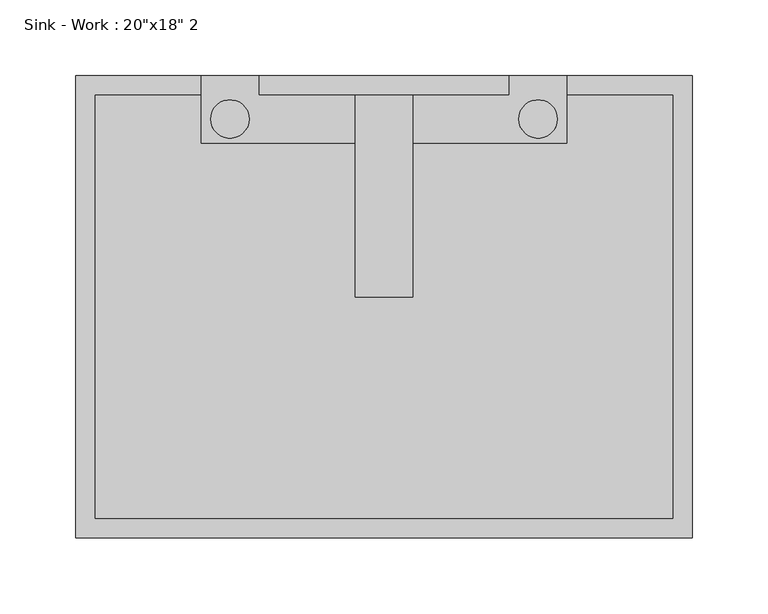
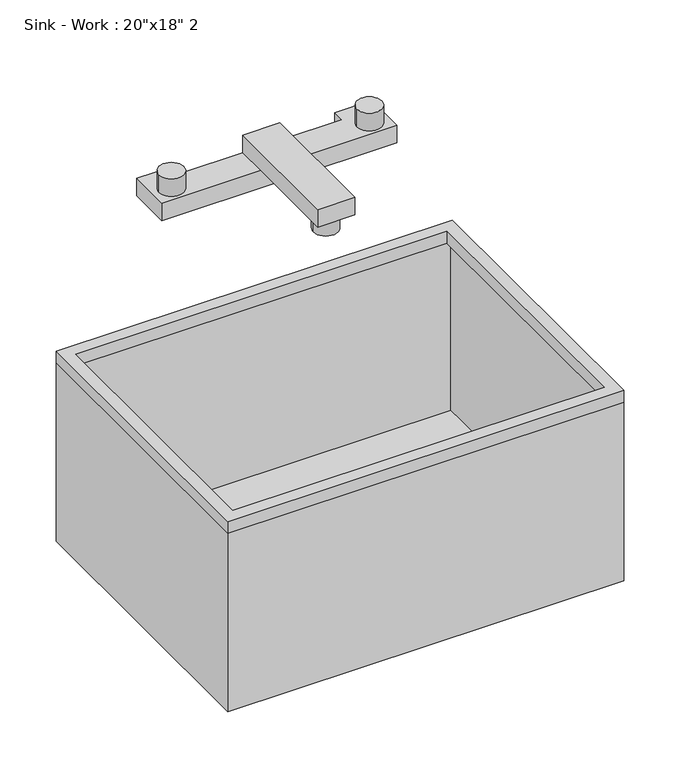
"""IFC4 building model written with IfcOpenShell, lengths in millimetres: flow terminal geometry."""

from ifc_helpers import new_model, si_unit, point, frame, frame_2d, origin, origin_with_axes, place, context, project, spatial, polyline, circle_curve, trimmed, segment, composite_curve, outline, extrude, faceted_brep, source, transform, mapped, element, save
from ifc_brep_helpers import plane_surface, cylinder_surface, advanced_brep


def flow_terminal_7145266d(model_context):
    return source(origin(), model_context, "Body", "SolidModel", [
        extrude(outline(polyline([(203.2, 0.0), (203.2, -304.8), (-203.2, -304.8), (-203.2, 0.0), (203.2, 0.0)]), holes=[polyline([(190.5, -12.7), (-190.5, -12.7), (-190.5, -292.1), (190.5, -292.1), (190.5, -12.7)])]), frame((0.0, 0.0, 193.675), z_axis=(0.0, 0.0, 1.0), x_axis=(1.0, 0.0, 0.0)), (0.0, 0.0, 1.0), 12.7),
        faceted_brep([(203.2, 0.0, 193.675), (-203.2, 0.0, 193.675), (-203.2, -304.8, 193.675), (203.2, -304.8, 193.675), (200.025, -3.175, 193.675), (200.025, -301.625, 193.675), (-200.025, -301.625, 193.675), (-200.025, -3.175, 193.675), (203.2, 0.0, 0.0), (203.2, -304.8, 0.0), (-203.2, -304.8, 0.0), (-203.2, 0.0, 0.0), (200.025, -3.175, 3.175), (200.025, -301.625, 3.175), (-200.025, -301.625, 3.175), (-200.025, -3.175, 3.175)], [[[0, 1, 2, 3], [4, 5, 6, 7]], [[8, 9, 10, 11]], [[1, 0, 8, 11]], [[2, 1, 11, 10]], [[3, 2, 10, 9]], [[0, 3, 9, 8]], [[5, 4, 12, 13]], [[6, 5, 13, 14]], [[7, 6, 14, 15]], [[4, 7, 15, 12]], [[13, 12, 15, 14]]]),
        extrude(outline(composite_curve([segment(trimmed(circle_curve(frame_2d((0.0, -127.0)), 25.4), [point((-25.4, -127.0))], [point((25.4, -127.0))], False, "CARTESIAN"), True, "CONTINUOUS"), segment(trimmed(circle_curve(frame_2d((0.0, -127.0)), 25.4), [point((25.4, -127.0))], [point((-25.4, -127.0))], False, "CARTESIAN"), True, "CONTINUOUS")], self_intersect=False)), origin_with_axes(), (0.0, 0.0, 1.0), 3.175),
        advanced_brep(
        [(19.05, -12.7, 384.175), (-19.05, -12.7, 384.175), (-19.05, -146.05, 384.175), (19.05, -146.05, 384.175), (19.05, -146.05, 365.125), (-19.05, -146.05, 365.125), (-19.05, -44.45, 365.125), (19.05, -44.45, 365.125), (-12.7, -127.0, 365.125), (12.7, -127.0, 365.125), (19.05, -12.7, 365.125), (82.55, -12.7, 365.125), (82.55, -12.7, 346.075), (-82.55, -12.7, 346.075), (-82.55, -12.7, 365.125), (-19.05, -12.7, 365.125), (-12.7, -127.0, 346.075), (12.7, -127.0, 346.075), (-82.55, 0.0, 365.125), (-120.65, 0.0, 365.125), (-120.65, -44.45, 365.125), (-88.9, -28.575, 365.125), (-114.3, -28.575, 365.125), (120.65, -44.45, 365.125), (120.65, 0.0, 365.125), (82.55, 0.0, 365.125), (114.3, -28.575, 365.125), (88.9, -28.575, 365.125), (-82.55, 0.0, 346.075), (82.55, 0.0, 346.075), (120.65, 0.0, 346.075), (120.65, -44.45, 346.075), (-120.65, -44.45, 346.075), (-120.65, 0.0, 346.075), (-114.3, -28.575, 384.175), (-88.9, -28.575, 384.175), (88.9, -28.575, 384.175), (114.3, -28.575, 384.175)],
        [
            (0, 1),
            (1, 2),
            (2, 3),
            (3, 0),
            (4, 5),
            (5, 6),
            (6, 7),
            (7, 4),
            (8, 9, circle_curve(frame((0.0, -127.0, 365.125), z_axis=(0.0, 0.0, 1.0), x_axis=(1.0, 0.0, 0.0)), 12.7)),
            (9, 8, circle_curve(frame((0.0, -127.0, 365.125), z_axis=(0.0, 0.0, 1.0), x_axis=(1.0, 0.0, 0.0)), 12.7)),
            (0, 10),
            (10, 11),
            (11, 12),
            (12, 13),
            (13, 14),
            (14, 15),
            (15, 1),
            (15, 6),
            (5, 2),
            (4, 3),
            (7, 10),
            (16, 17, circle_curve(frame((0.0, -127.0, 346.075), z_axis=(0.0, 0.0, -1.0), x_axis=(1.0, 0.0, 0.0)), 12.7)),
            (17, 16, circle_curve(frame((0.0, -127.0, 346.075), z_axis=(0.0, 0.0, -1.0), x_axis=(1.0, 0.0, 0.0)), 12.7)),
            (17, 9),
            (8, 16),
            (18, 19),
            (19, 20),
            (20, 6),
            (14, 18),
            (21, 22, circle_curve(frame((-101.6, -28.575, 365.125), z_axis=(0.0, 0.0, -1.0), x_axis=(1.0, 0.0, 0.0)), 12.7)),
            (22, 21, circle_curve(frame((-101.6, -28.575, 365.125), z_axis=(0.0, 0.0, -1.0), x_axis=(1.0, 0.0, 0.0)), 12.7)),
            (23, 24),
            (24, 25),
            (25, 11),
            (7, 23),
            (26, 27, circle_curve(frame((101.6, -28.575, 365.125), z_axis=(0.0, 0.0, -1.0), x_axis=(1.0, 0.0, 0.0)), 12.7)),
            (27, 26, circle_curve(frame((101.6, -28.575, 365.125), z_axis=(0.0, 0.0, -1.0), x_axis=(1.0, 0.0, 0.0)), 12.7)),
            (28, 13),
            (12, 29),
            (29, 30),
            (30, 31),
            (31, 32),
            (32, 33),
            (33, 28),
            (18, 28),
            (33, 19),
            (32, 20),
            (31, 23),
            (30, 24),
            (29, 25),
            (34, 35, circle_curve(frame((-101.6, -28.575, 384.175), z_axis=(0.0, 0.0, 1.0), x_axis=(1.0, 0.0, 0.0)), 12.7)),
            (35, 34, circle_curve(frame((-101.6, -28.575, 384.175), z_axis=(0.0, 0.0, 1.0), x_axis=(1.0, 0.0, 0.0)), 12.7)),
            (36, 37, circle_curve(frame((101.6, -28.575, 384.175), z_axis=(0.0, 0.0, 1.0), x_axis=(1.0, 0.0, 0.0)), 12.7)),
            (37, 36, circle_curve(frame((101.6, -28.575, 384.175), z_axis=(0.0, 0.0, 1.0), x_axis=(1.0, 0.0, 0.0)), 12.7)),
            (34, 22),
            (21, 35),
            (36, 27),
            (26, 37),
        ],
        [
            plane_surface(frame((-19.05, -12.7, 384.175), z_axis=(0.0, 0.0, 1.0), x_axis=(-1.0, 0.0, 0.0))),
            plane_surface(frame((-19.05, -12.7, 365.125), z_axis=(0.0, 0.0, -1.0), x_axis=(1.0, 0.0, 0.0))),
            plane_surface(frame((19.05, -12.7, 384.175), z_axis=(0.0, 1.0, 0.0), x_axis=(0.0, 0.0, -1.0))),
            plane_surface(frame((-19.05, -12.7, 384.175), z_axis=(-1.0, 0.0, 0.0), x_axis=(0.0, 0.0, -1.0))),
            plane_surface(frame((-19.05, -146.05, 384.175), z_axis=(0.0, -1.0, 0.0), x_axis=(0.0, 0.0, -1.0))),
            plane_surface(frame((19.05, -146.05, 384.175), z_axis=(1.0, 0.0, 0.0), x_axis=(0.0, 0.0, -1.0))),
            plane_surface(frame((12.7, -127.0, 346.075), z_axis=(0.0, 0.0, -1.0), x_axis=(0.0, -1.0, 0.0))),
            cylinder_surface(frame((0.0, -127.0, 346.075), z_axis=(0.0, 0.0, 1.0), x_axis=(1.0, 0.0, 0.0)), 12.7),
            plane_surface(frame((-120.65, 0.0, 365.125), z_axis=(0.0, 0.0, 1.0), x_axis=(-1.0, 0.0, 0.0))),
            plane_surface(frame((-120.65, 0.0, 346.075), z_axis=(0.0, 0.0, -1.0), x_axis=(1.0, 0.0, 0.0))),
            plane_surface(frame((-82.55, 0.0, 365.125), z_axis=(0.0, 1.0, 0.0), x_axis=(0.0, 0.0, -1.0))),
            plane_surface(frame((-120.65, 0.0, 365.125), z_axis=(-1.0, 0.0, 0.0), x_axis=(0.0, 0.0, -1.0))),
            plane_surface(frame((-120.65, -44.45, 365.125), z_axis=(0.0, -1.0, 0.0), x_axis=(0.0, 0.0, -1.0))),
            plane_surface(frame((120.65, -44.45, 365.125), z_axis=(1.0, 0.0, 0.0), x_axis=(0.0, 0.0, -1.0))),
            plane_surface(frame((120.65, 0.0, 365.125), z_axis=(0.0, 1.0, 0.0), x_axis=(0.0, 0.0, -1.0))),
            plane_surface(frame((82.55, 0.0, 365.125), z_axis=(-1.0, 0.0, 0.0), x_axis=(0.0, 0.0, -1.0))),
            plane_surface(frame((-82.55, -12.7, 365.125), z_axis=(1.0, 0.0, 0.0), x_axis=(0.0, 0.0, -1.0))),
            plane_surface(frame((-88.9, -28.575, 384.175), z_axis=(0.0, 0.0, 1.0), x_axis=(0.0, 1.0, 0.0))),
            cylinder_surface(frame((-101.6, -28.575, 365.125), z_axis=(0.0, 0.0, 1.0), x_axis=(1.0, 0.0, 0.0)), 12.7),
            cylinder_surface(frame((101.6, -28.575, 0.0), z_axis=(0.0, 0.0, 1.0), x_axis=(1.0, 0.0, 0.0)), 12.7),
        ],
        [
            (0, [[1, 2, 3, 4]]),
            (1, [[5, 6, 7, 8], [9, 10]]),
            (2, [[-1, 11, 12, 13, 14, 15, 16, 17]]),
            (3, [[-2, -17, 18, -6, 19]]),
            (4, [[-3, -19, -5, 20]]),
            (5, [[-4, -20, -8, 21, -11]]),
            (6, [[22, 23]]),
            (7, [[-23, 24, -9, 25]]),
            (7, [[-22, -25, -10, -24]]),
            (8, [[26, 27, 28, -18, -16, 29], [30, 31]]),
            (8, [[32, 33, 34, -12, -21, 35], [36, 37]]),
            (9, [[38, -14, 39, 40, 41, 42, 43, 44]]),
            (10, [[-26, 45, -44, 46]]),
            (11, [[-27, -46, -43, 47]]),
            (12, [[-42, 48, -35, -7, -28, -47]]),
            (13, [[-32, -48, -41, 49]]),
            (14, [[-33, -49, -40, 50]]),
            (15, [[-34, -50, -39, -13]]),
            (16, [[-29, -15, -38, -45]]),
            (17, [[51, 52]]),
            (17, [[53, 54]]),
            (18, [[-51, 55, -30, 56]]),
            (18, [[-52, -56, -31, -55]]),
            (19, [[-53, 57, -36, 58]]),
            (19, [[-54, -58, -37, -57]]),
        ],
    ),
    ])


if __name__ == "__main__":
    model = new_model("IFC4")
    model_context = context("Model", 3, world=origin())
    ifc_project = project(units=[si_unit("LENGTHUNIT", "METRE", prefix="MILLI")], contexts=[model_context])
    site = spatial("IfcSite", under=ifc_project)
    building = spatial("IfcBuilding", under=site)
    placement = place(None, origin())
    flow_terminal_shape = flow_terminal_7145266d(model_context)
    element("IfcFlowTerminal", 1, ObjectType="Sink - Work : 20\"x18\" 2", at=placement, inside=building, context=model_context, shape_type="MappedRepresentation", body=[
        mapped(flow_terminal_shape, transform((0.0, 0.0, 0.0), x_axis=(1.0, 0.0, 0.0), y_axis=(0.0, 1.0, 0.0), z_axis=(0.0, 0.0, 1.0))),
    ])
    save(model, "model.ifc")

# Revit data of these elements
# Type "Sink - Work : 20\"x18\" 2"
#   WFU = 2
#   Sink Width = 1' - 0"
#   Sink Length = 1' - 4"
#   Sink Depth = 0' - 8"
#   Sanitary Radius = 3/4"
#   Sanitary Diameter = 1 1/2"
#   Hot Water Radius = 1/4"
#   Hot Water Diameter = 1/2"
#   HWFU = 2.25
#   Flow Pressure [instance default] = 8.00 psi
#   Faucet Height = 1' - 1 5/8"
#   Cold Water Radius = 1/4"
#   Cold Water Diameter = 1/2"
#   CWFU = 2.25
#   Sink Material = none
#   Faucet Material = none
#   Default Elevation = 0
